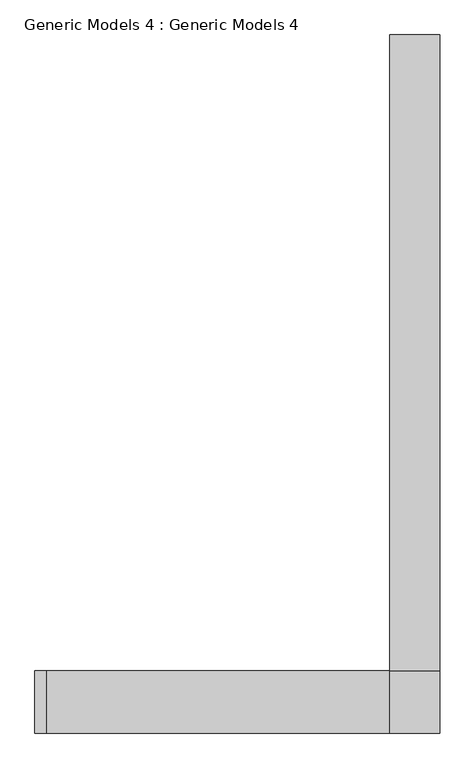
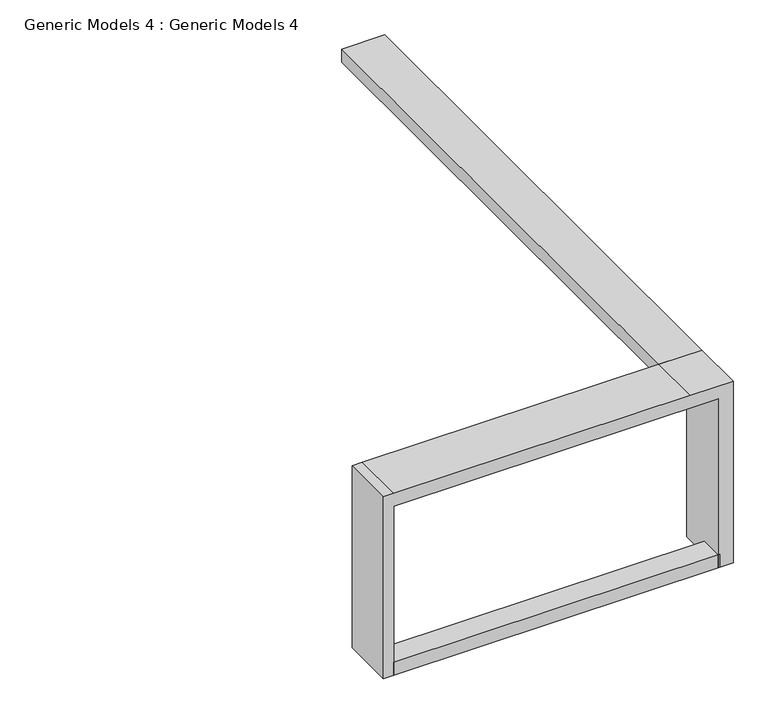
"""IFC4 building model written with IfcOpenShell, lengths in millimetres: proxy geometry, Generic Models 4 : Generic Models 4."""

from ifc_helpers import new_model, si_unit, frame, origin, place, context, project, spatial, polyline, outline, extrude, source, transform, mapped, element, save


def generic_models_4_generic_models_4_de5db2ce(model_context):
    return source(origin(), model_context, "Body", "SweptSolid", [
        extrude(outline(polyline([(-326.1740352, 1402.2984882), (-326.1740352, -10789.7015118), (-1278.9002751, -10789.7015118), (-1278.9002751, 1402.2984882), (-326.1740352, 1402.2984882)])), frame((0.0, 0.0, 3048.0), z_axis=(0.0, 0.0, 1.0), x_axis=(1.0, 0.0, 0.0)), (0.0, 0.0, 1.0), 304.8),
        extrude(outline(polyline([(-7860.2229687, -11987.6125482), (-7860.2229687, -11454.2125482), (-627.7343959, -11454.2125482), (-627.7343959, -11987.6125482), (-7860.2229687, -11987.6125482)])), frame((0.0, 0.0, -914.4), z_axis=(0.0, 0.0, 1.0), x_axis=(1.0, 0.0, 0.0)), (0.0, 0.0, 1.0), 304.8),
        extrude(outline(polyline([(3048.0, -7860.2229687), (3048.0, -659.3229687), (-914.4, -659.3229687), (-914.4, -326.1740352), (3352.8, -326.1740352), (3352.8, -1278.9002751), (3352.8, -7860.2229687), (3352.8, -8088.8229687), (-914.4, -8088.8229687), (-914.4, -7860.2229687), (3048.0, -7860.2229687)])), frame((0.0, -11987.6125482, 0.0), z_axis=(0.0, 1.0, 0.0), x_axis=(0.0, 0.0, 1.0)), (0.0, 0.0, 1.0), 1197.9110364),
    ])


if __name__ == "__main__":
    model = new_model("IFC4")
    model_context = context("Model", 3, world=origin())
    ifc_project = project(units=[si_unit("LENGTHUNIT", "METRE", prefix="MILLI")], contexts=[model_context])
    site = spatial("IfcSite", under=ifc_project)
    building = spatial("IfcBuilding", under=site)
    placement = place(None, origin())
    generic_models_4_generic_models_4_shape = generic_models_4_generic_models_4_de5db2ce(model_context)
    element("IfcBuildingElementProxy", 1, Name="Generic Models 4 : Generic Models 4", ObjectType="Generic Models 4 : Generic Models 4", at=placement, inside=building, context=model_context, shape_type="MappedRepresentation", body=[
        mapped(generic_models_4_generic_models_4_shape, transform((0.0, 0.0, 0.0), x_axis=(1.0, 0.0, 0.0), y_axis=(0.0, 1.0, 0.0), z_axis=(0.0, 0.0, 1.0))),
    ])
    save(model, "model.ifc")
